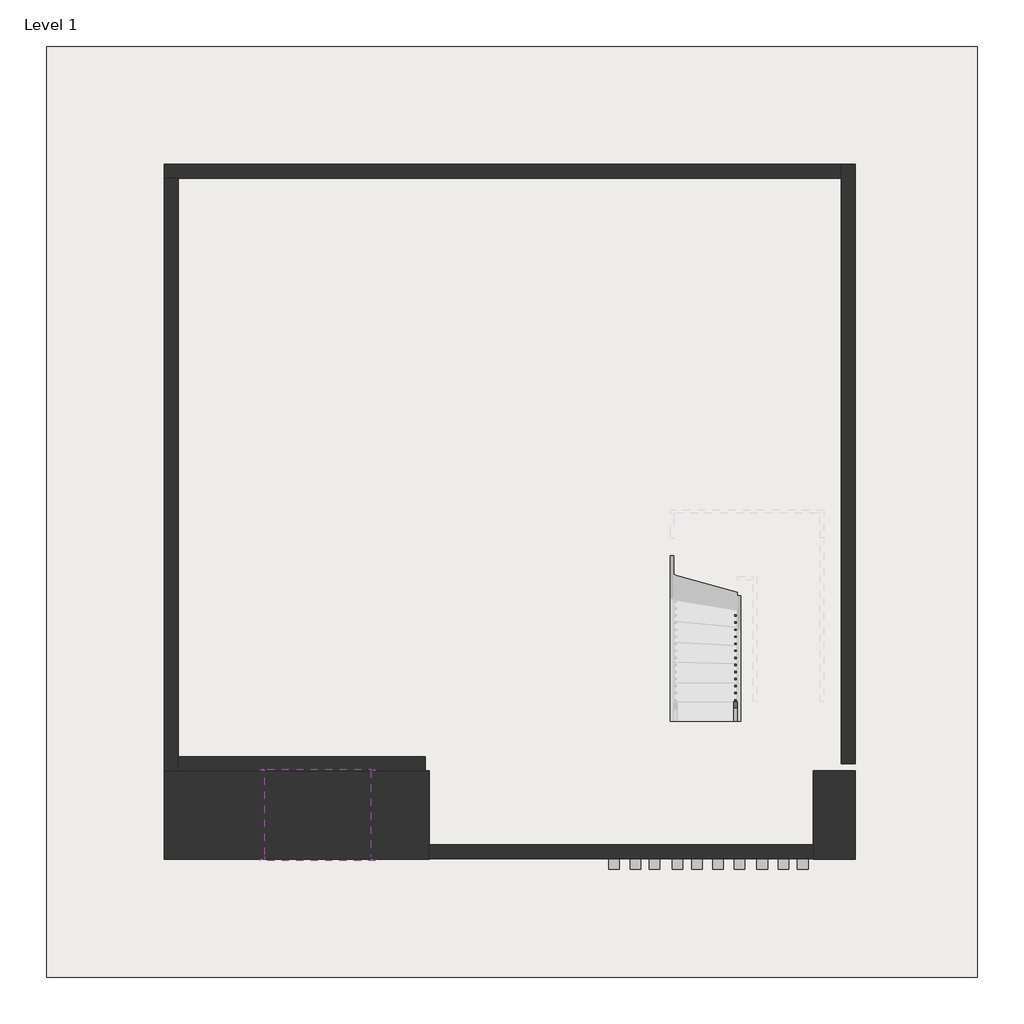
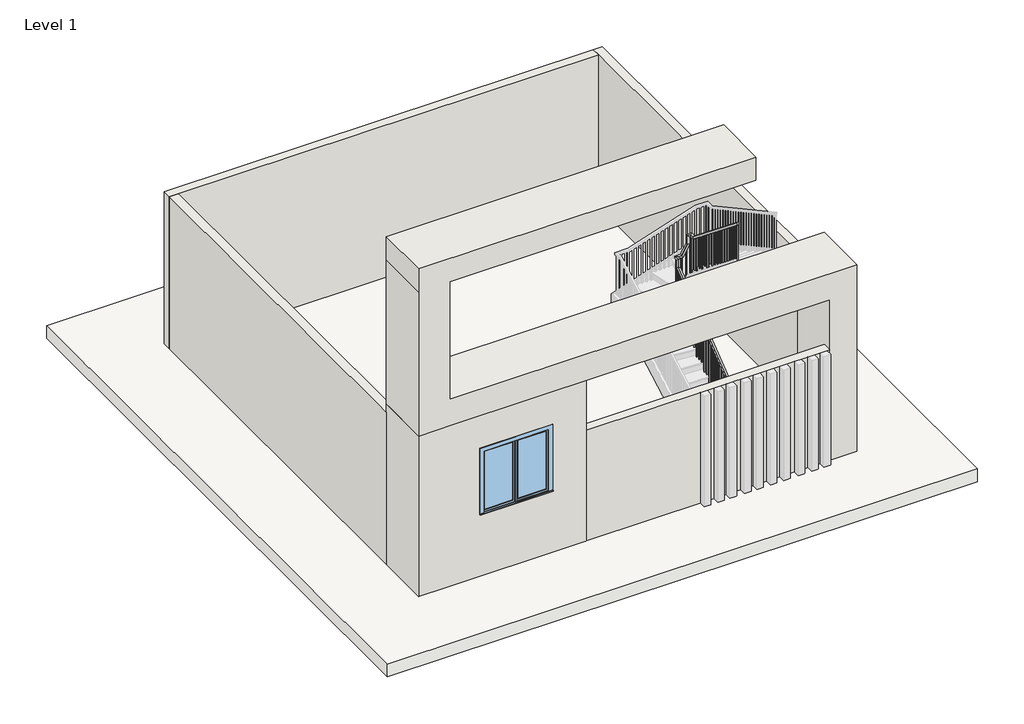
# One storey, part 1 of 2: 7 walls, 1 railing, 1 slab, 1 window.
"""IFC4 building model written with IfcOpenShell, lengths in millimetres."""

from ifc_helpers import new_model, si_unit, frame, origin, origin_with_axes, place, context, project, spatial, polyline, outline, extrude, faceted_brep, transform, mapped, element, save
from components import walls_1_walls_1_5b47a2ba, walls_2_walls_2_253db866, window_0f4f1f5f

model = new_model("IFC4")

# Units and contexts
model_context = context("Model", 3, world=origin())
ifc_project = project(units=[si_unit("LENGTHUNIT", "METRE", prefix="MILLI")], contexts=[model_context])

# Site, building, storey
site = spatial("IfcSite", under=ifc_project)
building = spatial("IfcBuilding", under=site)
storey = spatial("IfcBuildingStorey", under=building, Name="Level 1", Elevation=0.0)

# Railing
placement = place(None, origin())
element("IfcRailing", 1, ObjectType="Handrail - Rectangular", at=placement, inside=storey, context=model_context, shape_type="SolidModel", body=[
    faceted_brep([(-4608.9931367, 3267.4797066, 1047.0434898), (-4608.9931367, 3267.4797066, 982.8664163), (-4558.1931367, 3267.4797066, 982.8664163), (-4558.1931367, 3267.4797066, 1047.0434898), (-4608.9931367, 5277.8113984, 2599.0380287), (-4608.9931367, 5328.6113984, 2574.079022), (-4558.1931367, 5328.6113984, 2574.079022), (-4558.1931367, 5277.8113984, 2599.0380287), (-4608.9931367, 5277.8113984, 2805.8347079), (-4608.9931367, 5328.6113984, 2755.0347079), (-4558.1931367, 5328.6113984, 2755.0347079), (-4558.1931367, 5277.8113984, 2805.8347079), (-4608.9931367, 5404.8113984, 2805.8347079), (-4608.9931367, 5404.8113984, 2755.0347079), (-4558.1931367, 5354.0113984, 2755.0347079), (-4558.1931367, 5354.0113984, 2805.8347079), (-4481.9931367, 5404.8113984, 2805.8347079), (-4452.4586868, 5404.8113984, 2755.0347079), (-4452.4586868, 5354.0113984, 2755.0347079), (-4481.9931367, 5354.0113984, 2805.8347079), (-4354.9931367, 5404.8113984, 3028.9081493), (-4304.1931367, 5404.8113984, 3015.4607435), (-4304.1931367, 5354.0113984, 3015.4607435), (-4354.9931367, 5354.0113984, 3028.9081493), (-4354.9931367, 5404.8113984, 3237.7174934), (-4304.1931367, 5404.8113984, 3186.9174934), (-4304.1931367, 5354.0113984, 3186.9174934), (-4354.9931367, 5354.0113984, 3237.7174934), (-4227.9931367, 5404.8113984, 3237.7174934), (-4227.9931367, 5404.8113984, 3186.9174934), (-4278.7931367, 5354.0113984, 3186.9174934), (-4278.7931367, 5354.0113984, 3237.7174934), (-4227.9931367, 5277.8113984, 3237.7174934), (-4227.9931367, 5260.0050768, 3186.9174934), (-4278.7931367, 5260.0050768, 3186.9174934), (-4278.7931367, 5277.8113984, 3237.7174934), (-4227.9931367, 3546.8797066, 4621.1340886), (-4278.7931367, 3546.8797066, 4621.1340886), (-4278.7931367, 3546.8797066, 4556.1027004), (-4227.9931367, 3546.8797066, 4556.1027004)], [[[0, 1, 2, 3]], [[1, 0, 4, 5]], [[2, 1, 5, 6]], [[3, 2, 6, 7]], [[0, 3, 7, 4]], [[5, 4, 8, 9]], [[6, 5, 9, 10]], [[7, 6, 10, 11]], [[4, 7, 11, 8]], [[9, 8, 12, 13]], [[10, 9, 13, 14]], [[11, 10, 14, 15]], [[8, 11, 15, 12]], [[13, 12, 16, 17]], [[14, 13, 17, 18]], [[15, 14, 18, 19]], [[12, 15, 19, 16]], [[17, 16, 20, 21]], [[18, 17, 21, 22]], [[19, 18, 22, 23]], [[16, 19, 23, 20]], [[21, 20, 24, 25]], [[22, 21, 25, 26]], [[23, 22, 26, 27]], [[20, 23, 27, 24]], [[25, 24, 28, 29]], [[26, 25, 29, 30]], [[27, 26, 30, 31]], [[24, 27, 31, 28]], [[29, 28, 32, 33]], [[30, 29, 33, 34]], [[31, 30, 34, 35]], [[28, 31, 35, 32]], [[36, 37, 38, 39]], [[33, 32, 36, 39]], [[34, 33, 39, 38]], [[35, 34, 38, 37]], [[32, 35, 37, 36]]]),
    extrude(outline(polyline([(3610.8737375, 4504.956601), (3629.9237375, 4489.7312248), (3629.9237375, 3483.4285714), (3610.8737375, 3483.4285714), (3610.8737375, 4504.956601)])), frame((-4262.9181367, 0.0, 0.0), z_axis=(1.0, 0.0, 0.0), x_axis=(0.0, 1.0, 0.0)), (0.0, 0.0, 1.0), 19.05),
    extrude(outline(polyline([(3712.4737375, 4423.7545948), (3731.5237375, 4408.5292186), (3731.5237375, 3483.4285714), (3712.4737375, 3483.4285714), (3712.4737375, 4423.7545948)])), frame((-4262.9181367, 0.0, 0.0), z_axis=(1.0, 0.0, 0.0), x_axis=(0.0, 1.0, 0.0)), (0.0, 0.0, 1.0), 19.05),
    extrude(outline(polyline([(3814.0737375, 4342.5525885), (3833.1237375, 4327.3272123), (3833.1237375, 3483.4285714), (3814.0737375, 3483.4285714), (3814.0737375, 4342.5525885)])), frame((-4262.9181367, 0.0, 0.0), z_axis=(1.0, 0.0, 0.0), x_axis=(0.0, 1.0, 0.0)), (0.0, 0.0, 1.0), 19.05),
    extrude(outline(polyline([(3915.6737375, 4261.3505823), (3934.7237375, 4246.1252061), (3934.7237375, 3309.2571429), (3915.6737375, 3309.2571429), (3915.6737375, 4261.3505823)])), frame((-4262.9181367, 0.0, 0.0), z_axis=(1.0, 0.0, 0.0), x_axis=(0.0, 1.0, 0.0)), (0.0, 0.0, 1.0), 19.05),
    extrude(outline(polyline([(4017.2737375, 4180.148576), (4036.3237375, 4164.9231998), (4036.3237375, 3309.2571429), (4017.2737375, 3309.2571429), (4017.2737375, 4180.148576)])), frame((-4262.9181367, 0.0, 0.0), z_axis=(1.0, 0.0, 0.0), x_axis=(0.0, 1.0, 0.0)), (0.0, 0.0, 1.0), 19.05),
    extrude(outline(polyline([(4118.8737375, 4098.9465697), (4137.9237375, 4083.7211936), (4137.9237375, 3135.0857143), (4118.8737375, 3135.0857143), (4118.8737375, 4098.9465697)])), frame((-4262.9181367, 0.0, 0.0), z_axis=(1.0, 0.0, 0.0), x_axis=(0.0, 1.0, 0.0)), (0.0, 0.0, 1.0), 19.05),
    extrude(outline(polyline([(4220.4737375, 4017.7445635), (4239.5237375, 4002.5191873), (4239.5237375, 3135.0857143), (4220.4737375, 3135.0857143), (4220.4737375, 4017.7445635)])), frame((-4262.9181367, 0.0, 0.0), z_axis=(1.0, 0.0, 0.0), x_axis=(0.0, 1.0, 0.0)), (0.0, 0.0, 1.0), 19.05),
    extrude(outline(polyline([(4322.0737375, 3936.5425572), (4341.1237375, 3921.3171811), (4341.1237375, 3135.0857143), (4322.0737375, 3135.0857143), (4322.0737375, 3936.5425572)])), frame((-4262.9181367, 0.0, 0.0), z_axis=(1.0, 0.0, 0.0), x_axis=(0.0, 1.0, 0.0)), (0.0, 0.0, 1.0), 19.05),
    extrude(outline(polyline([(4423.6737375, 3855.340551), (4442.7237375, 3840.1151748), (4442.7237375, 2960.9142857), (4423.6737375, 2960.9142857), (4423.6737375, 3855.340551)])), frame((-4262.9181367, 0.0, 0.0), z_axis=(1.0, 0.0, 0.0), x_axis=(0.0, 1.0, 0.0)), (0.0, 0.0, 1.0), 19.05),
    extrude(outline(polyline([(4525.2737375, 3774.1385447), (4544.3237375, 3758.9131685), (4544.3237375, 2960.9142857), (4525.2737375, 2960.9142857), (4525.2737375, 3774.1385447)])), frame((-4262.9181367, 0.0, 0.0), z_axis=(1.0, 0.0, 0.0), x_axis=(0.0, 1.0, 0.0)), (0.0, 0.0, 1.0), 19.05),
    extrude(outline(polyline([(4626.8737375, 3692.9365385), (4645.9237375, 3677.7111623), (4645.9237375, 2786.7428571), (4626.8737375, 2786.7428571), (4626.8737375, 3692.9365385)])), frame((-4262.9181367, 0.0, 0.0), z_axis=(1.0, 0.0, 0.0), x_axis=(0.0, 1.0, 0.0)), (0.0, 0.0, 1.0), 19.05),
    extrude(outline(polyline([(4728.4737375, 3611.7345322), (4747.5237375, 3596.509156), (4747.5237375, 2786.7428571), (4728.4737375, 2786.7428571), (4728.4737375, 3611.7345322)])), frame((-4262.9181367, 0.0, 0.0), z_axis=(1.0, 0.0, 0.0), x_axis=(0.0, 1.0, 0.0)), (0.0, 0.0, 1.0), 19.05),
    extrude(outline(polyline([(4830.0737375, 3530.532526), (4849.1237375, 3515.3071498), (4849.1237375, 2786.7428571), (4830.0737375, 2786.7428571), (4830.0737375, 3530.532526)])), frame((-4262.9181367, 0.0, 0.0), z_axis=(1.0, 0.0, 0.0), x_axis=(0.0, 1.0, 0.0)), (0.0, 0.0, 1.0), 19.05),
    extrude(outline(polyline([(4931.6737375, 3449.3305197), (4950.7237375, 3434.1051435), (4950.7237375, 2612.5714286), (4931.6737375, 2612.5714286), (4931.6737375, 3449.3305197)])), frame((-4262.9181367, 0.0, 0.0), z_axis=(1.0, 0.0, 0.0), x_axis=(0.0, 1.0, 0.0)), (0.0, 0.0, 1.0), 19.05),
    extrude(outline(polyline([(5033.2737375, 3368.1285134), (5052.3237375, 3352.9031373), (5052.3237375, 2612.5714286), (5033.2737375, 2612.5714286), (5033.2737375, 3368.1285134)])), frame((-4262.9181367, 0.0, 0.0), z_axis=(1.0, 0.0, 0.0), x_axis=(0.0, 1.0, 0.0)), (0.0, 0.0, 1.0), 19.05),
    extrude(outline(polyline([(5134.8737375, 3286.9265072), (5153.9237375, 3271.701131), (5153.9237375, 2438.4), (5134.8737375, 2438.4), (5134.8737375, 3286.9265072)])), frame((-4262.9181367, 0.0, 0.0), z_axis=(1.0, 0.0, 0.0), x_axis=(0.0, 1.0, 0.0)), (0.0, 0.0, 1.0), 19.05),
    extrude(outline(polyline([(5236.4737375, 3205.7245009), (5255.5237375, 3190.4991248), (5255.5237375, 2438.4), (5236.4737375, 2438.4), (5236.4737375, 3205.7245009)])), frame((-4262.9181367, 0.0, 0.0), z_axis=(1.0, 0.0, 0.0), x_axis=(0.0, 1.0, 0.0)), (0.0, 0.0, 1.0), 19.05),
    extrude(outline(polyline([(2923.3962905, -4356.6072002), (2889.9352743, -4375.6572002), (1915.8857143, -4375.6572002), (1915.8857143, -4356.6072002), (2923.3962905, -4356.6072002)])), frame((0.0, 5369.8863984, 0.0), z_axis=(0.0, 1.0, 0.0), x_axis=(0.0, 0.0, 1.0)), (0.0, 0.0, 1.0), 19.05),
    extrude(outline(polyline([(2744.9375373, -4458.2072002), (2711.4765211, -4477.2572002), (1915.8857143, -4477.2572002), (1915.8857143, -4458.2072002), (2744.9375373, -4458.2072002)])), frame((0.0, 5369.8863984, 0.0), z_axis=(0.0, 1.0, 0.0), x_axis=(0.0, 0.0, 1.0)), (0.0, 0.0, 1.0), 19.05),
    extrude(outline(polyline([(5289.9547066, 2544.2357006), (5309.0047066, 2558.9424757), (5309.0047066, 1567.5428571), (5289.9547066, 1567.5428571), (5289.9547066, 2544.2357006)])), frame((-4593.1181367, 0.0, 0.0), z_axis=(1.0, 0.0, 0.0), x_axis=(0.0, 1.0, 0.0)), (0.0, 0.0, 1.0), 19.05),
    extrude(outline(polyline([(5188.3547066, 2465.799567), (5207.4047066, 2480.5063421), (5207.4047066, 1393.3714286), (5188.3547066, 1393.3714286), (5188.3547066, 2465.799567)])), frame((-4593.1181367, 0.0, 0.0), z_axis=(1.0, 0.0, 0.0), x_axis=(0.0, 1.0, 0.0)), (0.0, 0.0, 1.0), 19.05),
    extrude(outline(polyline([(5086.7547066, 2387.3634334), (5105.8047066, 2402.0702085), (5105.8047066, 1219.2), (5086.7547066, 1219.2), (5086.7547066, 2387.3634334)])), frame((-4593.1181367, 0.0, 0.0), z_axis=(1.0, 0.0, 0.0), x_axis=(0.0, 1.0, 0.0)), (0.0, 0.0, 1.0), 19.05),
    extrude(outline(polyline([(4985.1547066, 2308.9272998), (5004.2047066, 2323.6340749), (5004.2047066, 1219.2), (4985.1547066, 1219.2), (4985.1547066, 2308.9272998)])), frame((-4593.1181367, 0.0, 0.0), z_axis=(1.0, 0.0, 0.0), x_axis=(0.0, 1.0, 0.0)), (0.0, 0.0, 1.0), 19.05),
    extrude(outline(polyline([(4883.5547066, 2230.4911663), (4902.6047066, 2245.1979413), (4902.6047066, 1219.2), (4883.5547066, 1219.2), (4883.5547066, 2230.4911663)])), frame((-4593.1181367, 0.0, 0.0), z_axis=(1.0, 0.0, 0.0), x_axis=(0.0, 1.0, 0.0)), (0.0, 0.0, 1.0), 19.05),
    extrude(outline(polyline([(4781.9547066, 2152.0550327), (4801.0047066, 2166.7618077), (4801.0047066, 1045.0285714), (4781.9547066, 1045.0285714), (4781.9547066, 2152.0550327)])), frame((-4593.1181367, 0.0, 0.0), z_axis=(1.0, 0.0, 0.0), x_axis=(0.0, 1.0, 0.0)), (0.0, 0.0, 1.0), 19.05),
    extrude(outline(polyline([(4680.3547066, 2073.6188991), (4699.4047066, 2088.3256741), (4699.4047066, 1045.0285714), (4680.3547066, 1045.0285714), (4680.3547066, 2073.6188991)])), frame((-4593.1181367, 0.0, 0.0), z_axis=(1.0, 0.0, 0.0), x_axis=(0.0, 1.0, 0.0)), (0.0, 0.0, 1.0), 19.05),
    extrude(outline(polyline([(4578.7547066, 1995.1827655), (4597.8047066, 2009.8895405), (4597.8047066, 870.8571429), (4578.7547066, 870.8571429), (4578.7547066, 1995.1827655)])), frame((-4593.1181367, 0.0, 0.0), z_axis=(1.0, 0.0, 0.0), x_axis=(0.0, 1.0, 0.0)), (0.0, 0.0, 1.0), 19.05),
    extrude(outline(polyline([(4477.1547066, 1916.7466319), (4496.2047066, 1931.4534069), (4496.2047066, 870.8571429), (4477.1547066, 870.8571429), (4477.1547066, 1916.7466319)])), frame((-4593.1181367, 0.0, 0.0), z_axis=(1.0, 0.0, 0.0), x_axis=(0.0, 1.0, 0.0)), (0.0, 0.0, 1.0), 19.05),
    extrude(outline(polyline([(4375.5547066, 1838.3104983), (4394.6047066, 1853.0172733), (4394.6047066, 870.8571429), (4375.5547066, 870.8571429), (4375.5547066, 1838.3104983)])), frame((-4593.1181367, 0.0, 0.0), z_axis=(1.0, 0.0, 0.0), x_axis=(0.0, 1.0, 0.0)), (0.0, 0.0, 1.0), 19.05),
    extrude(outline(polyline([(4273.9547066, 1759.8743647), (4293.0047066, 1774.5811397), (4293.0047066, 696.6857143), (4273.9547066, 696.6857143), (4273.9547066, 1759.8743647)])), frame((-4593.1181367, 0.0, 0.0), z_axis=(1.0, 0.0, 0.0), x_axis=(0.0, 1.0, 0.0)), (0.0, 0.0, 1.0), 19.05),
    extrude(outline(polyline([(4172.3547066, 1681.4382311), (4191.4047066, 1696.1450061), (4191.4047066, 696.6857143), (4172.3547066, 696.6857143), (4172.3547066, 1681.4382311)])), frame((-4593.1181367, 0.0, 0.0), z_axis=(1.0, 0.0, 0.0), x_axis=(0.0, 1.0, 0.0)), (0.0, 0.0, 1.0), 19.05),
    extrude(outline(polyline([(4070.7547066, 1603.0020975), (4089.8047066, 1617.7088725), (4089.8047066, 522.5142857), (4070.7547066, 522.5142857), (4070.7547066, 1603.0020975)])), frame((-4593.1181367, 0.0, 0.0), z_axis=(1.0, 0.0, 0.0), x_axis=(0.0, 1.0, 0.0)), (0.0, 0.0, 1.0), 19.05),
    extrude(outline(polyline([(3969.1547066, 1524.5659639), (3988.2047066, 1539.2727389), (3988.2047066, 522.5142857), (3969.1547066, 522.5142857), (3969.1547066, 1524.5659639)])), frame((-4593.1181367, 0.0, 0.0), z_axis=(1.0, 0.0, 0.0), x_axis=(0.0, 1.0, 0.0)), (0.0, 0.0, 1.0), 19.05),
    extrude(outline(polyline([(3867.5547066, 1446.1298303), (3886.6047066, 1460.8366053), (3886.6047066, 522.5142857), (3867.5547066, 522.5142857), (3867.5547066, 1446.1298303)])), frame((-4593.1181367, 0.0, 0.0), z_axis=(1.0, 0.0, 0.0), x_axis=(0.0, 1.0, 0.0)), (0.0, 0.0, 1.0), 19.05),
    extrude(outline(polyline([(3765.9547066, 1367.6936967), (3785.0047066, 1382.4004718), (3785.0047066, 348.3428571), (3765.9547066, 348.3428571), (3765.9547066, 1367.6936967)])), frame((-4593.1181367, 0.0, 0.0), z_axis=(1.0, 0.0, 0.0), x_axis=(0.0, 1.0, 0.0)), (0.0, 0.0, 1.0), 19.05),
    extrude(outline(polyline([(3664.3547066, 1289.2575631), (3683.4047066, 1303.9643382), (3683.4047066, 348.3428571), (3664.3547066, 348.3428571), (3664.3547066, 1289.2575631)])), frame((-4593.1181367, 0.0, 0.0), z_axis=(1.0, 0.0, 0.0), x_axis=(0.0, 1.0, 0.0)), (0.0, 0.0, 1.0), 19.05),
    extrude(outline(polyline([(3562.7547066, 1210.8214295), (3581.8047066, 1225.5282046), (3581.8047066, 348.3428571), (3562.7547066, 348.3428571), (3562.7547066, 1210.8214295)])), frame((-4593.1181367, 0.0, 0.0), z_axis=(1.0, 0.0, 0.0), x_axis=(0.0, 1.0, 0.0)), (0.0, 0.0, 1.0), 19.05),
    extrude(outline(polyline([(3461.1547066, 1132.3852959), (3480.2047066, 1147.092071), (3480.2047066, 174.1714286), (3461.1547066, 174.1714286), (3461.1547066, 1132.3852959)])), frame((-4593.1181367, 0.0, 0.0), z_axis=(1.0, 0.0, 0.0), x_axis=(0.0, 1.0, 0.0)), (0.0, 0.0, 1.0), 19.05),
    extrude(outline(polyline([(3359.5547066, 1053.9491623), (3378.6047066, 1068.6559374), (3378.6047066, 174.1714286), (3359.5547066, 174.1714286), (3359.5547066, 1053.9491623)])), frame((-4593.1181367, 0.0, 0.0), z_axis=(1.0, 0.0, 0.0), x_axis=(0.0, 1.0, 0.0)), (0.0, 0.0, 1.0), 19.05),
    extrude(outline(polyline([(-4262.9181367, 5357.1237375), (-4243.8681367, 5357.1237375), (-4243.8681367, 5338.0737375), (-4262.9181367, 5338.0737375), (-4262.9181367, 5357.1237375)])), frame((0.0, 0.0, 2264.2285714), z_axis=(0.0, 0.0, 1.0), x_axis=(1.0, 0.0, 0.0)), (0.0, 0.0, 1.0), 922.688922),
    extrude(outline(polyline([(-4262.9181367, 5369.8863984), (-4262.9181367, 5388.9363984), (-4243.8681367, 5388.9363984), (-4243.8681367, 5369.8863984), (-4262.9181367, 5369.8863984)])), frame((0.0, 0.0, 2264.2285714), z_axis=(0.0, 0.0, 1.0), x_axis=(1.0, 0.0, 0.0)), (0.0, 0.0, 1.0), 922.688922),
    extrude(outline(polyline([(-4277.393481, 5369.8863984), (-4277.393481, 5388.9363984), (-4258.343481, 5388.9363984), (-4258.343481, 5369.8863984), (-4277.393481, 5369.8863984)])), frame((0.0, 0.0, 2090.0571429), z_axis=(0.0, 0.0, 1.0), x_axis=(1.0, 0.0, 0.0)), (0.0, 0.0, 1.0), 1096.8603506),
    extrude(outline(polyline([(-4578.8572002, 5369.8863984), (-4578.8572002, 5388.9363984), (-4559.8072002, 5388.9363984), (-4559.8072002, 5369.8863984), (-4578.8572002, 5369.8863984)])), frame((0.0, 0.0, 1741.7142857), z_axis=(0.0, 0.0, 1.0), x_axis=(1.0, 0.0, 0.0)), (0.0, 0.0, 1.0), 1013.3204221),
    extrude(outline(polyline([(-4574.0681367, 5369.8863984), (-4593.1181367, 5369.8863984), (-4593.1181367, 5388.9363984), (-4574.0681367, 5388.9363984), (-4574.0681367, 5369.8863984)])), frame((0.0, 0.0, 1567.5428571), z_axis=(0.0, 0.0, 1.0), x_axis=(1.0, 0.0, 0.0)), (0.0, 0.0, 1.0), 1187.4918507),
    extrude(outline(polyline([(-4574.0681367, 5337.439759), (-4593.1181367, 5337.439759), (-4593.1181367, 5356.489759), (-4574.0681367, 5356.489759), (-4574.0681367, 5337.439759)])), frame((0.0, 0.0, 1567.5428571), z_axis=(0.0, 0.0, 1.0), x_axis=(1.0, 0.0, 0.0)), (0.0, 0.0, 1.0), 1187.4918507),
    extrude(outline(polyline([(3546.8797066, 4556.1027004), (3565.9297066, 4540.8773242), (3565.9297066, 3483.4285714), (3546.8797066, 3483.4285714), (3546.8797066, 4556.1027004)])), frame((-4262.9181367, 0.0, 0.0), z_axis=(1.0, 0.0, 0.0), x_axis=(0.0, 1.0, 0.0)), (0.0, 0.0, 1.0), 19.05),
    extrude(outline(polyline([(3267.4797066, 982.8664163), (3286.5297066, 997.5731913), (3286.5297066, 174.1714286), (3267.4797066, 174.1714286), (3267.4797066, 982.8664163)])), frame((-4593.1181367, 0.0, 0.0), z_axis=(1.0, 0.0, 0.0), x_axis=(0.0, 1.0, 0.0)), (0.0, 0.0, 1.0), 19.05),
])

# Slab
element("IfcSlab", 2, ObjectType="Generic - 12\"", at=placement, inside=storey, context=model_context, shape_type="SweptSolid", body=[
    extrude(outline(polyline([(-1097.4679019, 12989.3544718), (-1097.4679019, -421.8455282), (-14508.6679019, -421.8455282), (-14508.6679019, 12989.3544718), (-1097.4679019, 12989.3544718)])), frame((0.0, 0.0, -304.8), z_axis=(0.0, 0.0, 1.0), x_axis=(1.0, 0.0, 0.0)), (0.0, 0.0, 1.0), 304.8),
])

# Walls
element("IfcWall", 3, ObjectType="Generic - 8\"", at=placement, inside=storey, context=model_context, shape_type="Brep", body=[
    faceted_brep([(-12813.1931367, 11090.6797066, 0.0), (-12609.9931367, 11090.6797066, 0.0), (-3059.5931367, 11090.6797066, 0.0), (-3059.5931367, 11090.6797066, 3657.6), (-12609.9931367, 11090.6797066, 3657.6), (-12813.1931367, 11090.6797066, 3657.6), (-12813.1931367, 11293.8797066, 0.0), (-12813.1931367, 11293.8797066, 3657.6), (-3059.5931367, 11293.8797066, 3657.6), (-3059.5931367, 11293.8797066, 0.0)], [[[0, 1, 2, 3, 4, 5]], [[6, 7, 8, 9]], [[2, 1, 0, 6, 9]], [[0, 5, 7, 6]], [[3, 2, 9, 8]], [[5, 4, 3, 8, 7]]]),
])
element("IfcWall", 4, ObjectType="Generic - 8\"", at=placement, inside=storey, context=model_context, shape_type="Brep", body=[
    faceted_brep([(-12609.9931367, 2556.2797066, 0.0), (-12609.9931367, 2759.4797066, 0.0), (-12609.9931367, 11090.6797066, 0.0), (-12609.9931367, 11090.6797066, 3657.6), (-12609.9931367, 2759.4797066, 3657.6), (-12609.9931367, 2556.2797066, 3657.6), (-12813.1931367, 2556.2797066, 0.0), (-12813.1931367, 2556.2797066, 3657.6), (-12813.1931367, 11090.6797066, 3657.6), (-12813.1931367, 11090.6797066, 0.0)], [[[0, 1, 2, 3, 4, 5]], [[6, 7, 8, 9]], [[2, 1, 0, 6, 9]], [[0, 5, 7, 6]], [[3, 2, 9, 8]], [[5, 4, 3, 8, 7]]]),
])
element("IfcWall", 5, ObjectType="Generic - 8\"", at=placement, inside=storey, context=model_context, shape_type="SweptSolid", body=[
    extrude(outline(polyline([(-12609.9931367, 2759.4797066), (-9053.9931367, 2759.4797066), (-9053.9931367, 2556.2797066), (-12609.9931367, 2556.2797066), (-12609.9931367, 2759.4797066)])), origin_with_axes(), (0.0, 0.0, 1.0), 3657.6),
])
element("IfcWall", 6, ObjectType="Generic - 8\"", at=placement, inside=storey, context=model_context, shape_type="Brep", body=[
    faceted_brep([(-3059.5931367, 11293.8797066, 0.0), (-3059.5931367, 11090.6797066, 0.0), (-3059.5931367, 2657.8797066, 0.0), (-3059.5931367, 2657.8797066, 3657.6), (-3059.5931367, 11090.6797066, 3657.6), (-3059.5931367, 11293.8797066, 3657.6), (-2856.3931367, 11293.8797066, 0.0), (-2856.3931367, 11293.8797066, 3657.6), (-2856.3931367, 2657.8797066, 3657.6), (-2856.3931367, 2657.8797066, 0.0)], [[[0, 1, 2, 3, 4, 5]], [[6, 7, 8, 9]], [[2, 1, 0, 6, 9]], [[3, 2, 9, 8]], [[0, 5, 7, 6]], [[5, 4, 3, 8, 7]]]),
])
element("IfcWall", 7, ObjectType="Generic - 8\"", at=placement, inside=storey, context=model_context, shape_type="SweptSolid", body=[
    extrude(outline(polyline([(-3465.9931367, 1286.2797066), (-8998.6105967, 1286.2797066), (-8998.6105967, 1489.4797066), (-3465.9931367, 1489.4797066), (-3465.9931367, 1286.2797066)])), origin_with_axes(), (0.0, 0.0, 1.0), 2659.145604),
])
walls_1_walls_1_shape = walls_1_walls_1_5b47a2ba(model_context)
element("IfcWall", 8, ObjectType="Walls 1 : Walls 1", at=placement, inside=storey, context=model_context, shape_type="MappedRepresentation", body=[
    mapped(walls_1_walls_1_shape, transform((0.0, 0.0, 0.0), x_axis=(1.0, 0.0, 0.0), y_axis=(0.0, 1.0, 0.0), z_axis=(0.0, 0.0, 1.0))),
])
walls_2_walls_2_shape = walls_2_walls_2_253db866(model_context)
element("IfcWall", 9, ObjectType="Walls 2 : Walls 2", at=placement, inside=storey, context=model_context, shape_type="MappedRepresentation", body=[
    mapped(walls_2_walls_2_shape, transform((0.0, 0.0, 0.0), x_axis=(1.0, 0.0, 0.0), y_axis=(0.0, 1.0, 0.0), z_axis=(0.0, 0.0, 1.0))),
])

# Window
window_shape = window_0f4f1f5f(model_context)
element("IfcWindow", 10, ObjectType="Casement Dbl with Trim.0001 : 60\" x 60\"", at=placement, inside=storey, context=model_context, shape_type="MappedRepresentation", body=[
    mapped(window_shape, transform((-10600.5013745, 1938.2768481, 570.0102642), x_axis=(-1.0, 0.0, 0.0), y_axis=(0.0, -1.0, 0.0), z_axis=(0.0, 0.0, 1.0))),
])

save(model, "model.ifc")

# Revit data of these elements
# Type "Handrail - Rectangular"
#   Assembly Code = "C2010400"
#   built-in parameter 1008612 = 0.0416667 (stored number, unit not read)
#   built-in parameter 1008611 = 0.0416667 (stored number, unit not read)
#   built-in parameter 1008609 = 0.333333 (stored number, unit not read)
#   built-in parameter 1008604 = 0.166667 (stored number, unit not read)
#   built-in parameter 1008603 = 0.166667 (stored number, unit not read)
#   Railing Height = 3' - 0"
#   built-in parameter 1008630 = 2
#   built-in parameter 1008610 = 2
#   built-in parameter 1008618 = Baluster - Square : 3/4"
# Type "Generic - 12\""
#   Assembly Code = "B1010"
#   Function = 0
#   Layers, outside or top first: 1' - 0" no material (function 1)
# Type "Generic - 8\""
#   Assembly Code = "B2010"
#   Layers, outside or top first: 0' - 8" no material (function 1)
# Type "Casement Dbl with Trim.0001 : 60\" x 60\""
#   Type Mark = "10"
#   Construction Type Id = "GSP4R"
#   Assembly Code = "B2020100"
#   Analytic Construction = "1/8 in Pilkington single glazing"
#   Visual Light Transmittance = 0.9
#   Solar Heat Gain Coefficient = 0.78
#   Heat Transfer Coefficient (U) = 0.6496 BTU/(h·ft²·°F)
#   Height = 5' - 0"
#   Default Sill Height = 3' - 0"
#   Trim Projection - Ext. = 0' - 0 1/2"
#   Trim Projection - Int. = 0' - 0 3/4"
#   Trim Width - Exterior = 0' - 3 1/2"
#   Trim Width - Interior = 0' - 3 1/2"
#   Width = 5' - 0"
#   Window Inset = 0' - 0 3/4"
#   Define Thermal Properties by = 1
#   Glass Pane Material = Glass
#   Sash Material = Sash
#   Trim Exterior Material = Trim
#   Trim Interior Material = Trim
#   Wall Closure = (empty or 0)
# Element 1 (IfcRailing, "Handrail - Rectangular")
#   Phase Created = New Construction
# Element 2 (IfcSlab, "Generic - 12\"")
#   Height Offset From Level = 0' - 0"
#   Phase Created = New Construction
#   Materials on its faces: "Default Floor"
# Elements 3, 4, 5, 6 (IfcWall, "Generic - 8\"")
#   Top Offset = 0' - 0"
#   Base Offset = 0' - 0"
#   Unconnected Height = 12' - 0"
#   wall height = 12' - 0"
#   Phase Created = New Construction
#   Base Constraint = Level 1
#   Materials on its faces: "Default Wall"
# Element 7 (IfcWall, "Generic - 8\"")
#   Top Offset = 0' - 0"
#   Base Offset = 0' - 0"
#   Unconnected Height = 8' - 8.69077"
#   wall height = 8' - 8.69077"
#   Phase Created = New Construction
#   Base Constraint = Level 1
#   Materials on its faces: "Default Wall"
# Element 8 (IfcWall, "Walls 1 : Walls 1")
#   Phase Created = New Construction
#   Materials on its faces: "Default Wall"
# Element 9 (IfcWall, "Walls 2 : Walls 2")
#   Phase Created = New Construction
#   Materials on its faces: "Default Wall"
# Element 10 (IfcWindow, "Casement Dbl with Trim.0001 : 60\" x 60\"")
#   Mark = "1"
#   Phase Created = New Construction
#   Materials on its faces: "Sash", "Trim", "Glass"
# Materials
#   "Glass": class "Glass", colour RGB 0 128 192, transparency 0.75, Description = "Soda Lime Glass", Cost = 0
#   "Sash": class "Wood", colour RGB 224 178 126, transparency 0
#   "Trim": class "Wood", colour RGB 224 178 126, transparency 0
#   "Default Floor": colour RGB 128 128 128, transparency 0
#   "Default Wall": colour RGB 128 128 128, transparency 0
